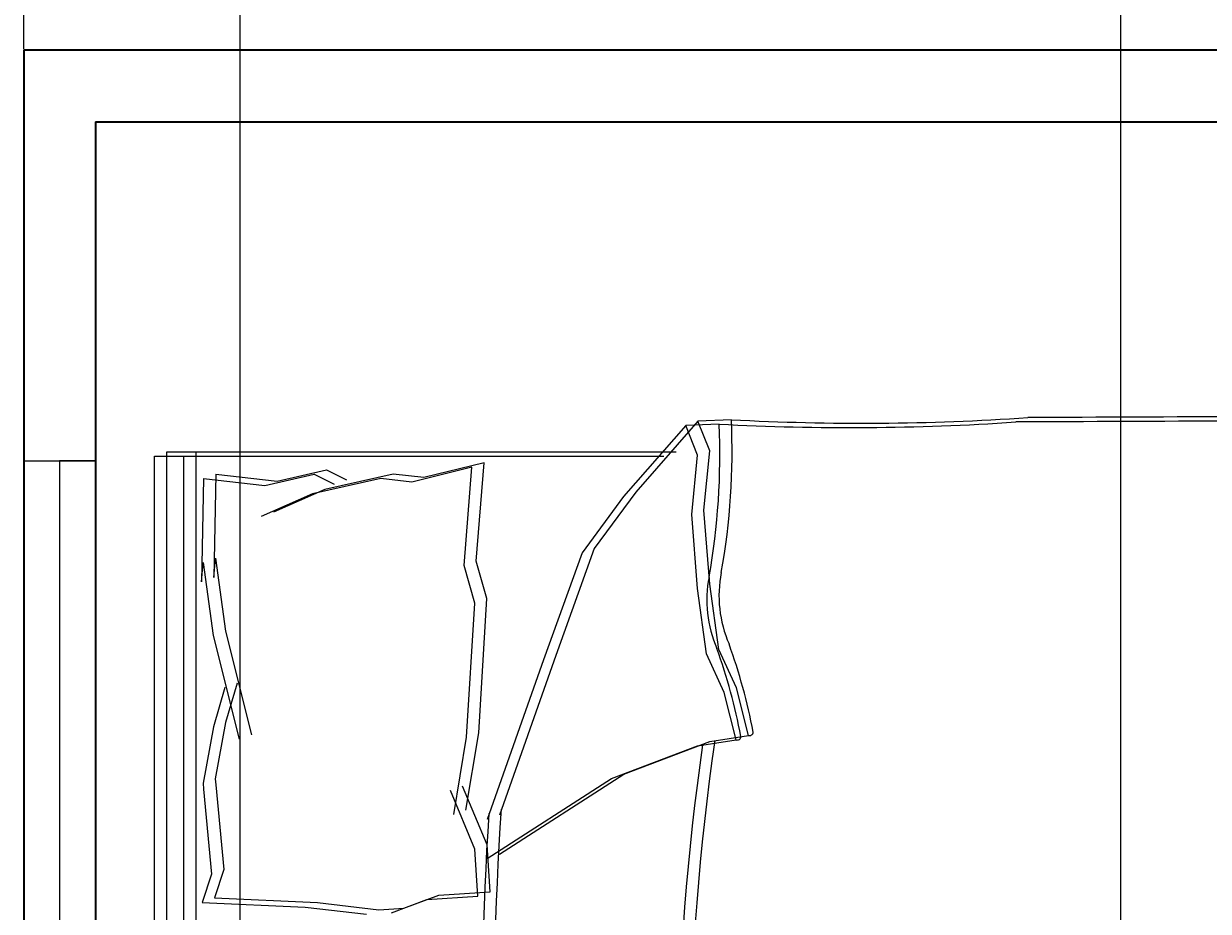
# Model space of a CAD drawing. Units: inches. Extents: x 1088 to 1703, y 668 to 1875.
# Tile 16 of 45: x 1170 to 1245, y 1750 to 1805. Entities that reach past the tile are written whole.
import ezdxf

# ---------------------------------------------------------------- set-up
doc = ezdxf.new("R2010")
doc.units = ezdxf.units.IN
for name, color, linetype, lineweight in [('A-ANNO-DIMS', 2, 'Continuous', 18), ('A-FURN', 8, 'Continuous', 13), ('A-GLAZ', 4, 'Continuous', 18), ('A-WALL', 7, 'Continuous', 35)]:
    doc.layers.add(name, color=color, linetype=linetype, lineweight=lineweight)
doc.styles.get("Standard").update_dxf_attribs({"font": 'arial.ttf'})
doc.dimstyles.get("Standard").update_dxf_attribs({"dimtxt": 0.18, "dimasz": 0.18, "dimexe": 0.18, "dimexo": 0.0625, "dimgap": 0.09, "dimtad": 0, "dimtih": 1, "dimtoh": 1, "dimdec": 4, "dimzin": 0, "dimdsep": 46, "dimtxsty": 'Standard', "dimcen": 0.09, "dimadec": 0, "dimazin": 0, "dimtfac": 1, "dimtdec": 4, "dimtofl": 0, "dimtmove": 0, "dimatfit": 3, "dimfxl": 1, "dimtolj": 1, "dimtzin": 0, "dimarcsym": 0})

# ---------------------------------------------------------------- blocks, each defined once
blk = doc.blocks.new('BED-DOUBLE')
for p, q in [((33.263, 63.381), (29.367, 58.939)), ((34.03, 63.655), (30.133, 59.213)), ((35.355, 63.476), (33.263, 63.381, 4.641)), ((34.006, 61.538), (33.263, 63.381)), ((36.121, 63.75), (34.03, 63.655, 4.641)), ((34.772, 61.812), (34.03, 63.655)), ((0.766, 61.734), (32.668, 61.734)), ((0.766, 4.44), (0.766, 61.734)), ((2.605, 4.44), (2.605, 61.734)), ((34.401, 58.099), (34.772, 61.812)), ((0, 61.46), (31.901, 61.46)), ((0, 4.167), (0, 61.46)), ((1.838, 4.167), (1.838, 61.46)), ((20.635, 61.054), (16.872, 60.124)), ((20.151, 54.902), (20.635, 61.054)), ((33.634, 57.825), (34.006, 61.538)), ((3.065, 60.077), (2.949, 53.601)), ((3.065, 60.077), (6.915, 59.624)), ((3.832, 60.351), (3.716, 53.875)), ((3.832, 60.351), (7.681, 59.897)), ((6.915, 59.624), (9.996, 60.337)), ((7.681, 59.897), (10.763, 60.611)), ((14.181, 60.078), (9.899, 59.115)), ((9.996, 60.337), (11.251, 59.721)), ((14.947, 60.351), (10.665, 59.389)), ((10.763, 60.611), (12.017, 59.995)), ((16.105, 59.851), (14.181, 60.078)), ((16.872, 60.124), (14.947, 60.351)), ((19.868, 60.78), (16.105, 59.851)), ((19.384, 54.628), (19.868, 60.78)), ((10.665, 59.389), (7.454, 57.973)), ((9.899, 59.115), (6.688, 57.699)), ((29.367, 58.939), (26.769, 55.411)), ((30.133, 59.213), (27.535, 55.685)), ((34.772, 53.457), (34.401, 58.099)), ((34.006, 53.183), (33.634, 57.825)), ((27.535, 55.685), (25.123, 49.001)), ((3.716, 53.875), (3.814, 55.077)), ((3.814, 55.077), (4.446, 50.523)), ((20.819, 52.552), (20.151, 54.902)), ((26.769, 55.411), (24.357, 48.727)), ((2.949, 53.601), (3.048, 54.803)), ((3.048, 54.803), (3.68, 50.25)), ((20.052, 52.278), (19.384, 54.628)), ((35.329, 49.372), (34.772, 53.457)), ((34.562, 49.098), (34.006, 53.183)), ((19.536, 43.874), (20.052, 52.278)), ((20.302, 44.148), (20.819, 52.552)), ((4.446, 50.523), (6.068, 44.027)), ((3.68, 50.25), (5.301, 43.753)), ((25.123, 49.001), (21.606, 39.005)), ((35.676, 46.685), (34.562, 49.098)), ((36.442, 46.958), (35.329, 49.372)), ((24.357, 48.727), (20.84, 38.731)), ((4.404, 46.996), (3.69, 44.52)), ((5.171, 47.27), (4.457, 44.794)), ((37.184, 43.988), (36.442, 46.958)), ((36.418, 43.714), (35.676, 46.685)), ((3.69, 44.52), (3.042, 41.007)), ((4.457, 44.794), (3.808, 41.281)), ((18.736, 39.04), (19.536, 43.874)), ((19.503, 39.314), (20.302, 44.148)), ((34.772, 43.616), (37.184, 43.988)), ((28.624, 41.3), (34.006, 43.342)), ((29.391, 41.574), (34.772, 43.616)), ((34.006, 43.342), (36.418, 43.714)), ((21.606, 36.551), (29.391, 41.574)), ((3.042, 41.007), (3.066, 40.622)), ((3.808, 41.281), (3.832, 40.896)), ((3.832, 40.896), (4.338, 35.587)), ((20.835, 37.139), (19.294, 40.82)), ((20.84, 36.277), (28.624, 41.3)), ((3.066, 40.622), (3.571, 35.314)), ((20.068, 36.866), (18.528, 40.547)), ((21.018, 34.199), (20.835, 37.139)), ((20.252, 33.925), (20.068, 36.866)), ((3.571, 35.314), (2.987, 33.541)), ((4.338, 35.587), (3.754, 33.814)), ((17.81, 33.998), (21.018, 34.199)), ((2.987, 33.541), (9.432, 33.249)), ((3.754, 33.814), (10.198, 33.523)), ((10.198, 33.523), (14.047, 33.069)), ((14.838, 32.892), (17.044, 33.725)), ((15.604, 33.166), (17.81, 33.998)), ((17.044, 33.725), (20.252, 33.925)), ((9.432, 33.249), (13.281, 32.795)), ((14.047, 33.069), (15.604, 33.166))]:
    blk.add_line(p, q)
for centre, radius, start, end in [((44.303, 218.785), 155.251, 266.97912, 273.83645), ((82.075, -5405.068), 5469.019, 90.002168, 90.286887), ((-7.98, 61.534), 43.378, 349.87628, 2.56571), ((43.537, 218.511), 155.251, 266.97912, 273.83645), ((-7.213, 61.808), 43.378, 349.87628, 2.56571), ((81.308, -5405.342), 5469.019, 90.002168, 90.286887), ((42.806, 52.716), 7.462, 168.6608, 203.73842), ((42.039, 52.443), 7.462, 168.6608, 203.73842), ((2.543, 37.623), 35.551, 10.66171, 19.88058), ((1.777, 37.349), 35.551, 10.66171, 19.88058), ((36.492, 43.922), 0.221, 250.24637, 1.13765), ((37.259, 44.196), 0.221, 250.24637, 1.13765), ((187.401, 21.287), 154.676, 171.78449, 186.90062), ((188.167, 21.561), 154.676, 171.78449, 186.90062), ((219.021, 25.88), 197.774, 176.08655, 186.78213), ((218.255, 25.607), 197.774, 176.08655, 186.78213)]:
    blk.add_arc(centre, radius, start, end)
blk = doc.blocks.new('*D28')
at = {"layer": 'A-ANNO-DIMS', "color": 0, "lineweight": -2, "transparency": 16777216}
for p, q in [((1170.345, 1803.621), (1170.345, 1857.788)), ((1170.525, 1857.608), (1408.147, 1857.608)), ((1646.563, 1857.608), (1408.941, 1857.608)), ((1646.743, 1745.552), (1646.743, 1857.788))]:
    blk.add_line(p, q, dxfattribs=at)
at = {"layer": 'A-ANNO-DIMS', "color": 0, "transparency": 16777216}
for points in [[(1170.525, 1857.638), (1170.525, 1857.578), (1170.345, 1857.608)], [(1646.563, 1857.638), (1646.563, 1857.578), (1646.743, 1857.608)]]:
    blk.add_solid(points, dxfattribs=at)
at = {"layer": 'Defpoints', "color": 0, "transparency": 16777216}
for p in [(1646.743, 1857.608), (1170.345, 1803.558), (1646.743, 1745.49)]:
    blk.add_point(p, dxfattribs=at)
at = {"layer": 'A-ANNO-DIMS', "color": 0, "transparency": 16777216, "insert": (1408.544, 1857.608), "char_height": 0.18, "attachment_point": 5}
blk.add_mtext('\\A1;476.4', dxfattribs=at)
blk = doc.blocks.new('*D35')
at = {"layer": 'A-ANNO-DIMS', "color": 0, "lineweight": -2, "transparency": 16777216}
for p, q in [((1183.893, 1448.103), (1183.893, 1857.788)), ((1184.073, 1857.608), (1211.072, 1857.608)), ((1238.859, 1857.608), (1211.86, 1857.608)), ((1239.039, 1448.103), (1239.039, 1857.788))]:
    blk.add_line(p, q, dxfattribs=at)
at = {"layer": 'A-ANNO-DIMS', "color": 0, "transparency": 16777216}
for points in [[(1184.073, 1857.638), (1184.073, 1857.578), (1183.893, 1857.608)], [(1238.859, 1857.638), (1238.859, 1857.578), (1239.039, 1857.608)]]:
    blk.add_solid(points, dxfattribs=at)
at = {"layer": 'Defpoints', "color": 0, "transparency": 16777216}
for p in [(1239.039, 1857.608), (1183.893, 1448.04), (1239.039, 1448.04)]:
    blk.add_point(p, dxfattribs=at)
at = {"layer": 'A-ANNO-DIMS', "color": 0, "transparency": 16777216, "insert": (1211.466, 1857.608), "char_height": 0.18, "attachment_point": 5}
blk.add_mtext('\\A1;55.15', dxfattribs=at)

msp = doc.modelspace()

# ---------------------------------------------------------------- linework, layer by layer
at = {"layer": 'A-GLAZ'}
for p, q in [((1170.345, 1777.837), (1174.845, 1777.837)), ((1174.845, 1777.837), (1172.595, 1777.837)), ((1172.595, 1777.837), (1172.595, 1717.837))]:
    msp.add_line(p, q, dxfattribs=at)
at = {"layer": 'A-WALL'}
for p, q in [((1170.345, 1803.558), (1317.345, 1803.558)), ((1170.345, 1803.558), (1317.345, 1803.558)), ((1170.345, 1803.558), (1317.345, 1803.558)), ((1170.345, 1803.558), (1317.345, 1803.558)), ((1170.345, 1803.558), (1317.345, 1803.558)), ((1170.345, 1803.558), (1170.345, 836.058)), ((1174.845, 1799.058), (1174.845, 1649.058)), ((1174.845, 1799.058), (1312.845, 1799.058))]:
    msp.add_line(p, q, dxfattribs=at)

# ---------------------------------------------------------------- block references
at = {"layer": 'A-FURN'}
msp.add_blockref('BED-DOUBLE', (1178.533, 1716.657), dxfattribs=at)

# ---------------------------------------------------------------- dimensions: what is measured, and where the dimension line sits
at = {"layer": 'A-ANNO-DIMS'}
for base, p1, p2, override, picture, middle in [((1646.743, 1857.608), (1170.345, 1803.558), (1646.743, 1745.49), {"dimdec": 1, "dimlfac": 1, "dimrnd": 0, "dimzin": 0, "dimdsep": 46, "dimlunit": 2}, '*D28', (1408.544, 1857.608)), ((1239.039, 1857.608), (1183.893, 1448.04), (1239.039, 1448.04), {"dimdec": 2, "dimlfac": 1, "dimrnd": 0, "dimzin": 0, "dimdsep": 46, "dimlunit": 2}, '*D35', (1211.466, 1857.608))]:
    dim = msp.add_linear_dim(base=base, p1=p1, p2=p2, dimstyle='Standard', override=override, dxfattribs=at)
    dim.commit()
    dim.dimension.update_dxf_attribs({"geometry": picture, "text_midpoint": middle})

doc.saveas('drawing.dxf')
